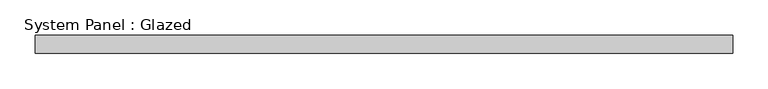
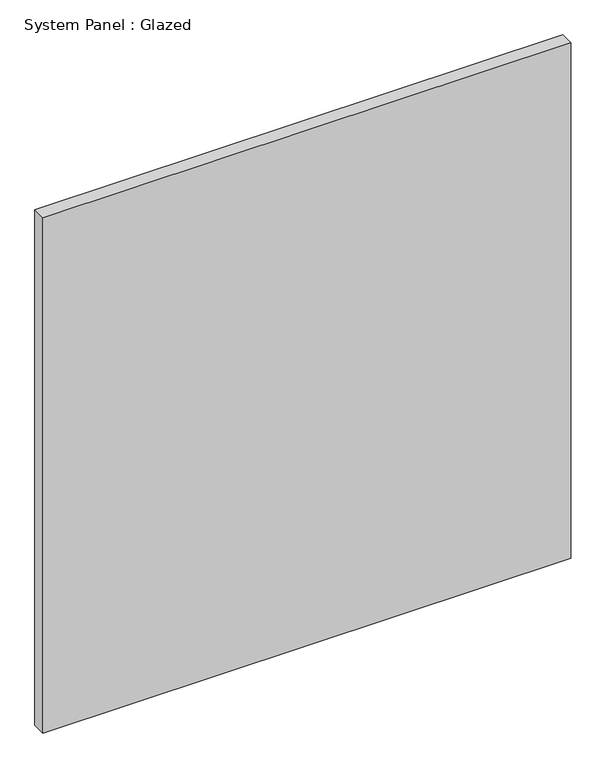
"""IFC4 building model written with IfcOpenShell, lengths in millimetres: plate geometry, System Panel : Glazed."""

from ifc_helpers import new_model, si_unit, origin, origin_with_axes, place, context, project, spatial, polyline, outline, extrude, source, transform, mapped, element, save


def system_panel_glazed_77e7111d(model_context):
    return source(origin(), model_context, "Body", "SweptSolid", [
        extrude(outline(polyline([(492.1956338, 19.05), (-492.1956338, 19.05), (-492.1956338, 44.45), (492.1956338, 44.45), (492.1956338, 19.05)])), origin_with_axes(), (0.0, 0.0, 1.0), 1016.2501856),
    ])


if __name__ == "__main__":
    model = new_model("IFC4")
    model_context = context("Model", 3, world=origin())
    ifc_project = project(units=[si_unit("LENGTHUNIT", "METRE", prefix="MILLI")], contexts=[model_context])
    site = spatial("IfcSite", under=ifc_project)
    building = spatial("IfcBuilding", under=site)
    placement = place(None, origin())
    system_panel_glazed_shape = system_panel_glazed_77e7111d(model_context)
    element("IfcPlate", 1, ObjectType="System Panel : Glazed", at=placement, inside=building, context=model_context, shape_type="MappedRepresentation", body=[
        mapped(system_panel_glazed_shape, transform((0.0, 0.0, 0.0), x_axis=(1.0, 0.0, 0.0), y_axis=(0.0, 1.0, 0.0), z_axis=(0.0, 0.0, 1.0))),
    ])
    save(model, "model.ifc")

# Revit data of these elements
# Type "System Panel : Glazed"
#   Construction Type Id = "GSP4R"
#   Analytic Construction = "1/8 in Pilkington single glazing"
#   Visual Light Transmittance = 0.9
#   Solar Heat Gain Coefficient = 0.86
#   Heat Transfer Coefficient (U) = 1.18115 BTU/(h·ft²·°F)
#   Define Thermal Properties by = 1
# Element 1 (IfcPlate, "System Panel : Glazed")
#   Materials on its faces: "Glass"
# Materials
#   "Glass": class "Glass", colour RGB 0 128 192, transparency 0.75, Description = "Soda Lime Glass", Cost = 0
